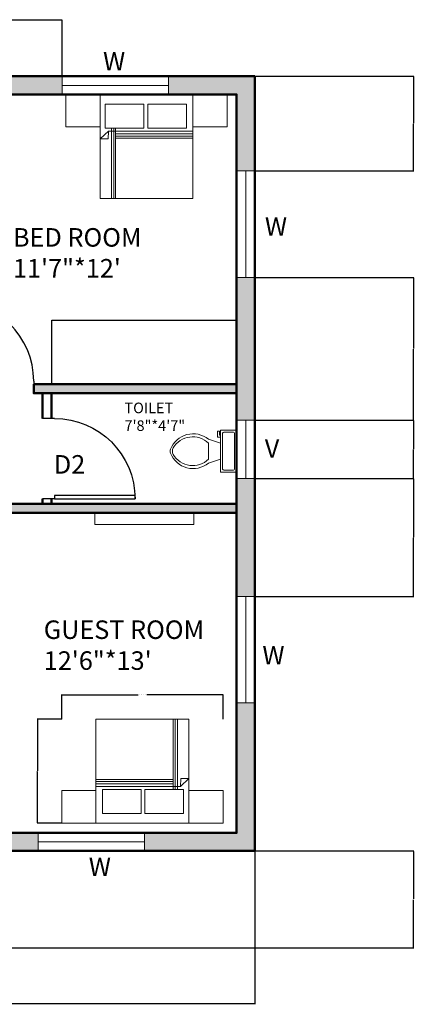
# Model space of a CAD drawing. Units: inches. Extents: x 2116 to 2704, y 2001 to 2561.
# Tile 2 of 2: x 2508 to 2704, y 2001 to 2490. Entities that reach past the tile are written whole.
import ezdxf

# ---------------------------------------------------------------- set-up
doc = ezdxf.new("R2010")
doc.units = ezdxf.units.IN
doc.linetypes.add('ACAD_ISO02W100', pattern=[15, 12, -3])
for name, color, linetype, lineweight in [('A-ANNO-DIMS', 2, 'Continuous', 18), ('A-AREA-IDEN', 70, 'Continuous', 25), ('A-DOOR', 3, 'Continuous', 25), ('A-FLOR-CASE', 9, 'Continuous', 25), ('A-FLOR-FIXT', 9, 'Continuous', 18), ('A-FURN', 40, 'Continuous', 18), ('A-GLAZ', 4, 'Continuous', 20), ('A-GLAZ-HIDN', 4, 'ACAD_ISO02W100', 18), ('A-WALL-PATT', 172, 'Continuous', 13), ('TEXT', 70, 'Continuous', 18), ('TV', 210, 'Continuous', 18), ('WALL', 7, 'Continuous', 50)]:
    doc.layers.add(name, color=color, linetype=linetype, lineweight=lineweight)
doc.styles.get("Standard").update_dxf_attribs({"font": 'arial.ttf'})
doc.dimstyles.get("Standard").update_dxf_attribs({"dimtxt": 0.18, "dimasz": 0.18, "dimexe": 0.18, "dimexo": 0.0625, "dimgap": 0.09, "dimtad": 0, "dimtih": 1, "dimtoh": 1, "dimdec": 4, "dimzin": 0, "dimdsep": 46, "dimtxsty": 'Standard', "dimcen": 0.09, "dimadec": 0, "dimazin": 0, "dimtfac": 1, "dimtdec": 4, "dimtofl": 0, "dimtmove": 0, "dimatfit": 3, "dimfxl": 1, "dimtolj": 1, "dimtzin": 0, "dimarcsym": 0})

# ---------------------------------------------------------------- blocks, each defined once
blk = doc.blocks.new('*U2')
for p, q in [((0, 0), (0, -6)), ((40, 0), (40, -6))]:
    blk.add_line(p, q)
blk.add_lwpolyline([(0, 0), (0, 40), (1.75, 40), (1.75, 0)], close=True)
blk.add_arc((0, 0), 40, 0, 90)
blk = doc.blocks.new('*U4')
for p, q in [((9.5, -6), (9.5, -2)), ((-10, -8.5), (-8, -8.5)), ((-10, -9.5), (-10, -8.5)), ((-7, -9.5), (-10, -9.5)), ((-8, -8.5), (-8, -8)), ((-7, -8), (-7, -9.5)), ((-4, -8), (-6, -14)), ((4, -8), (6, -14)), ((4, -14), (-4, -14))]:
    blk.add_line(p, q)
blk.add_lwpolyline([(10.5, -8), (10.5, 0), (-10.5, 0), (-10.5, -8)], close=True)
for points in [[(-9.5, -2), (-9.5, -6)], [(8.5, -1), (-8.5, -1)], [(-8.5, -7), (8.5, -7)]]:
    blk.add_lwpolyline(points)
for centre, radius, start, end in [((-8.62, -1.88), 0.884, 81.8699, 188.1301), ((8.62, -1.88), 0.884, 351.8699, 98.1301), ((-8.62, -6.12), 0.884, 171.8699, 278.1301), ((8.62, -6.12), 0.884, 261.8699, 8.1301), ((3.52, -21.58), 12.17, 141.4691, 247.9714), ((4.2, -21.82), 11.33, 136.3677, 238.9468), ((-3.52, -21.58), 12.17, 292.0284, 38.5307), ((-4.2, -21.82), 11.33, 301.053, 43.6321), ((0, -27.88), 4, 245.7318, 294.2682), ((0, -29), 4, 254.8605, 285.1395)]:
    blk.add_arc(centre, radius, start, end)
blk = doc.blocks.new('BED-DOUBLE-WITH-NIGHTSTANDS')
for p, q in [((22.66, 34.94), (22.66, 0)), ((23.77, 34.94), (23.77, 0)), ((24.74, 34.94), (24.74, 0)), ((21.16, 33.51), (16.99, 29.58)), ((16.99, 29.58), (21.04, 29.58)), ((21.04, 29.58), (21.16, 33.51)), ((63.16, 33.51), (21.16, 33.51)), ((24.74, 32.21), (63.16, 32.21)), ((24.74, 30.97), (63.16, 30.97)), ((24.74, 30.05), (63.16, 30.05))]:
    blk.add_line(p, q)
for points in [[(16.99, 51.74), (0, 51.74), (0, 35.55), (16.99, 35.55)], [(16.99, 51.74), (63.16, 51.74), (63.16, 0), (16.99, 0)], [(80.15, 51.74), (63.16, 51.74), (63.16, 35.55), (80.15, 35.55)], [(19.62, 46.86), (38.84, 46.86), (38.84, 34.94), (19.62, 34.94)], [(40.77, 46.86), (59.99, 46.86), (59.99, 34.94), (40.77, 34.94)]]:
    blk.add_lwpolyline(points, close=True)
blk = doc.blocks.new('WIN-PLAN-53IN-NOM')
blk.add_line((0, 4.5), (52.88, 4.5))
blk.add_lwpolyline([(0, 9), (52.88, 9), (52.88, 0), (0, 0)], close=True)
blk = doc.blocks.new('*D9')
at = {"layer": 'A-ANNO-DIMS', "color": 0, "lineweight": -2, "transparency": 16777216}
for p, q in [((2528.83, 2142.83), (2528.83, 2154.97)), ((2529.01, 2154.79), (2566.8, 2154.79)), ((2608.8, 2154.79), (2571.02, 2154.79)), ((2608.98, 2142.83), (2608.98, 2154.97))]:
    blk.add_line(p, q, dxfattribs=at)
at = {"layer": 'A-ANNO-DIMS', "color": 0, "lineweight": 100, "transparency": 16777216}
for points in [[(2529.01, 2154.82), (2529.01, 2154.76), (2528.83, 2154.79)], [(2608.8, 2154.82), (2608.8, 2154.76), (2608.98, 2154.79)]]:
    blk.add_solid(points, dxfattribs=at)
at = {"layer": 'Defpoints', "color": 0, "lineweight": 100, "transparency": 16777216}
for p in [(2528.83, 2154.79), (2528.83, 2142.77), (2608.98, 2142.77)]:
    blk.add_point(p, dxfattribs=at)
at = {"layer": 'A-ANNO-DIMS', "color": 0, "transparency": 16777216, "insert": (2568.91, 2154.79), "char_height": 0.18, "attachment_point": 5}
blk.add_mtext('\\A1;BED WITH NIGHTSTANDS 80 TYP.', dxfattribs=at)
blk = doc.blocks.new('*D10')
at = {"layer": 'A-ANNO-DIMS', "color": 0, "lineweight": -2, "transparency": 16777216}
for p, q in [((2528.77, 2142.77), (2516.63, 2142.77)), ((2516.81, 2142.59), (2516.81, 2117.08)), ((2516.81, 2091.21), (2516.81, 2116.72)), ((2528.77, 2091.03), (2516.63, 2091.03))]:
    blk.add_line(p, q, dxfattribs=at)
at = {"layer": 'A-ANNO-DIMS', "color": 0, "lineweight": 100, "transparency": 16777216}
for points in [[(2516.78, 2142.59), (2516.84, 2142.59), (2516.81, 2142.77)], [(2516.78, 2091.21), (2516.84, 2091.21), (2516.81, 2091.03)]]:
    blk.add_solid(points, dxfattribs=at)
at = {"layer": 'Defpoints', "color": 0, "lineweight": 100, "transparency": 16777216}
for p in [(2528.83, 2142.77), (2516.81, 2091.03), (2528.83, 2091.03)]:
    blk.add_point(p, dxfattribs=at)
at = {"layer": 'A-ANNO-DIMS', "color": 0, "transparency": 16777216, "insert": (2516.81, 2116.9), "char_height": 0.18, "attachment_point": 5}
blk.add_mtext('\\A1;52 TYP.', dxfattribs=at)
blk = doc.blocks.new('*D15')
at = {"layer": 'A-ANNO-DIMS', "color": 0, "lineweight": -2, "transparency": 16777216}
for p, q in [((2439.1, 2462.31), (2439.1, 2490.37)), ((2439.28, 2490.19), (2483.65, 2490.19)), ((2528.8, 2490.19), (2484.43, 2490.19)), ((2528.98, 2462.31), (2528.98, 2490.37))]:
    blk.add_line(p, q, dxfattribs=at)
at = {"layer": 'A-ANNO-DIMS', "color": 0, "lineweight": 100, "transparency": 16777216}
for points in [[(2439.28, 2490.22), (2439.28, 2490.16), (2439.1, 2490.19)], [(2528.8, 2490.22), (2528.8, 2490.16), (2528.98, 2490.19)]]:
    blk.add_solid(points, dxfattribs=at)
at = {"layer": 'Defpoints', "color": 0, "lineweight": 100, "transparency": 16777216}
for p in [(2528.98, 2490.19), (2439.1, 2462.24), (2528.98, 2462.24)]:
    blk.add_point(p, dxfattribs=at)
at = {"layer": 'A-ANNO-DIMS', "color": 0, "transparency": 16777216, "insert": (2484.04, 2490.19), "char_height": 0.18, "attachment_point": 5}
blk.add_mtext('\\A1;89.88', dxfattribs=at)
blk = doc.blocks.new('*D16')
at = {"layer": 'A-ANNO-DIMS', "color": 0, "lineweight": -2, "transparency": 16777216}
for p, q in [((2144.72, 2077.18), (2144.72, 2001.04)), ((2624.72, 2077.18), (2624.72, 2001.04)), ((2144.9, 2001.22), (2384.43, 2001.22)), ((2624.54, 2001.22), (2385.01, 2001.22))]:
    blk.add_line(p, q, dxfattribs=at)
at = {"layer": 'A-ANNO-DIMS', "color": 0, "lineweight": 100, "transparency": 16777216}
for points in [[(2144.9, 2001.25), (2144.9, 2001.19), (2144.72, 2001.22)], [(2624.54, 2001.25), (2624.54, 2001.19), (2624.72, 2001.22)]]:
    blk.add_solid(points, dxfattribs=at)
at = {"layer": 'Defpoints', "color": 0, "lineweight": 100, "transparency": 16777216}
for p in [(2144.72, 2077.24), (2624.72, 2077.24), (2624.72, 2001.22)]:
    blk.add_point(p, dxfattribs=at)
at = {"layer": 'A-ANNO-DIMS', "color": 0, "transparency": 16777216, "insert": (2384.72, 2001.22), "char_height": 0.18, "attachment_point": 5}
blk.add_mtext('\\A1;480', dxfattribs=at)
blk = doc.blocks.new('*D17')
at = {"layer": 'A-ANNO-DIMS', "color": 0, "lineweight": -2, "transparency": 16777216}
for p, q in [((2624.78, 2462.24), (2703.85, 2462.24)), ((2703.67, 2462.06), (2703.67, 2438.9)), ((2703.67, 2415.37), (2703.67, 2438.54)), ((2624.78, 2415.19), (2703.85, 2415.19))]:
    blk.add_line(p, q, dxfattribs=at)
at = {"layer": 'A-ANNO-DIMS', "color": 0, "lineweight": 100, "transparency": 16777216}
for points in [[(2703.64, 2462.06), (2703.7, 2462.06), (2703.67, 2462.24)], [(2703.64, 2415.37), (2703.7, 2415.37), (2703.67, 2415.19)]]:
    blk.add_solid(points, dxfattribs=at)
at = {"layer": 'Defpoints', "color": 0, "lineweight": 100, "transparency": 16777216}
for p in [(2624.72, 2462.24), (2703.67, 2462.24), (2624.72, 2415.19)]:
    blk.add_point(p, dxfattribs=at)
at = {"layer": 'A-ANNO-DIMS', "color": 0, "transparency": 16777216, "insert": (2703.67, 2438.72), "char_height": 0.18, "attachment_point": 5}
blk.add_mtext('\\A1;47.05', dxfattribs=at)
blk = doc.blocks.new('*D18')
at = {"layer": 'A-ANNO-DIMS', "color": 0, "lineweight": -2, "transparency": 16777216}
for p, q in [((2624.78, 2362.32), (2703.85, 2362.32)), ((2703.67, 2362.14), (2703.67, 2327.04)), ((2703.67, 2291.59), (2703.67, 2326.68)), ((2624.78, 2291.41), (2703.85, 2291.41))]:
    blk.add_line(p, q, dxfattribs=at)
at = {"layer": 'A-ANNO-DIMS', "color": 0, "lineweight": 100, "transparency": 16777216}
for points in [[(2703.64, 2362.14), (2703.7, 2362.14), (2703.67, 2362.32)], [(2703.64, 2291.59), (2703.7, 2291.59), (2703.67, 2291.41)]]:
    blk.add_solid(points, dxfattribs=at)
at = {"layer": 'Defpoints', "color": 0, "lineweight": 100, "transparency": 16777216}
for p in [(2624.72, 2362.32), (2703.67, 2362.32), (2624.72, 2291.41)]:
    blk.add_point(p, dxfattribs=at)
at = {"layer": 'A-ANNO-DIMS', "color": 0, "transparency": 16777216, "insert": (2703.67, 2326.86), "char_height": 0.18, "attachment_point": 5}
blk.add_mtext('\\A1;70.9', dxfattribs=at)
blk = doc.blocks.new('*D19')
at = {"layer": 'A-ANNO-DIMS', "color": 0, "lineweight": -2, "transparency": 16777216}
for p, q in [((2624.78, 2291.41), (2703.85, 2291.41)), ((2703.67, 2291.23), (2703.67, 2277.06)), ((2703.67, 2262.53), (2703.67, 2276.7)), ((2624.78, 2262.35), (2703.85, 2262.35))]:
    blk.add_line(p, q, dxfattribs=at)
at = {"layer": 'A-ANNO-DIMS', "color": 0, "lineweight": 100, "transparency": 16777216}
for points in [[(2703.64, 2291.23), (2703.7, 2291.23), (2703.67, 2291.41)], [(2703.64, 2262.53), (2703.7, 2262.53), (2703.67, 2262.35)]]:
    blk.add_solid(points, dxfattribs=at)
at = {"layer": 'Defpoints', "color": 0, "lineweight": 100, "transparency": 16777216}
for p in [(2624.72, 2291.41), (2703.67, 2291.41), (2624.72, 2262.35)]:
    blk.add_point(p, dxfattribs=at)
at = {"layer": 'A-ANNO-DIMS', "color": 0, "transparency": 16777216, "insert": (2703.67, 2276.88), "char_height": 0.18, "attachment_point": 5}
blk.add_mtext('\\A1;29.064', dxfattribs=at)
blk = doc.blocks.new('*D20')
at = {"layer": 'A-ANNO-DIMS', "color": 0, "lineweight": -2, "transparency": 16777216}
for p, q in [((2624.78, 2262.35), (2703.85, 2262.35)), ((2703.67, 2262.17), (2703.67, 2233.24)), ((2703.67, 2203.96), (2703.67, 2232.88)), ((2624.78, 2203.78), (2703.85, 2203.78))]:
    blk.add_line(p, q, dxfattribs=at)
at = {"layer": 'A-ANNO-DIMS', "color": 0, "lineweight": 100, "transparency": 16777216}
for points in [[(2703.64, 2262.17), (2703.7, 2262.17), (2703.67, 2262.35)], [(2703.64, 2203.96), (2703.7, 2203.96), (2703.67, 2203.78)]]:
    blk.add_solid(points, dxfattribs=at)
at = {"layer": 'Defpoints', "color": 0, "lineweight": 100, "transparency": 16777216}
for p in [(2624.72, 2262.35), (2703.67, 2262.35), (2624.72, 2203.78)]:
    blk.add_point(p, dxfattribs=at)
at = {"layer": 'A-ANNO-DIMS', "color": 0, "transparency": 16777216, "insert": (2703.67, 2233.06), "char_height": 0.18, "attachment_point": 5}
blk.add_mtext('\\A1;58.57', dxfattribs=at)
blk = doc.blocks.new('*D21')
at = {"layer": 'A-ANNO-DIMS', "color": 0, "lineweight": -2, "transparency": 16777216}
for p, q in [((2624.78, 2077.24), (2703.85, 2077.24)), ((2703.67, 2077.06), (2703.67, 2053.39)), ((2703.67, 2029.35), (2703.67, 2053.03)), ((2413.8, 2029.17), (2703.85, 2029.17))]:
    blk.add_line(p, q, dxfattribs=at)
at = {"layer": 'A-ANNO-DIMS', "color": 0, "lineweight": 100, "transparency": 16777216}
for points in [[(2703.64, 2077.06), (2703.7, 2077.06), (2703.67, 2077.24)], [(2703.64, 2029.35), (2703.7, 2029.35), (2703.67, 2029.17)]]:
    blk.add_solid(points, dxfattribs=at)
at = {"layer": 'Defpoints', "color": 0, "lineweight": 100, "transparency": 16777216}
for p in [(2624.72, 2077.24), (2703.67, 2077.24), (2413.74, 2029.17)]:
    blk.add_point(p, dxfattribs=at)
at = {"layer": 'A-ANNO-DIMS', "color": 0, "transparency": 16777216, "insert": (2703.67, 2053.21), "char_height": 0.18, "attachment_point": 5}
blk.add_mtext('\\A1;48.07', dxfattribs=at)

msp = doc.modelspace()

# ---------------------------------------------------------------- hatches: boundary and pattern name
at = {"layer": 'A-WALL-PATT'}
h = msp.add_hatch(color=256, dxfattribs=at)
h.dxf.hatch_style = 1
h.paths.add_polyline_path([(2187.7856, 2462.2434), (2144.722, 2462.2434), (2144.722, 2419.3525), (2153.722, 2419.3525), (2153.722, 2453.2434), (2187.7856, 2453.2434)])
h.paths.add_polyline_path([(2302.9116, 2462.2434), (2240.6643, 2462.2434), (2240.6643, 2453.2434), (2241.4366, 2453.2434), (2285.722, 2453.2434), (2302.9116, 2453.2434)])
h.paths.add_polyline_path([(2153.722, 2366.4738), (2144.722, 2366.4738), (2144.722, 2275.9883), (2153.722, 2275.9883)])
h.paths.add_polyline_path([(2386.2219, 2462.2434), (2332.038, 2462.2434), (2332.038, 2453.2434), (2344.222, 2453.2434), (2386.2219, 2453.2434)])
h.paths.add_polyline_path([(2528.9791, 2462.2434), (2439.1006, 2462.2434), (2439.1006, 2453.2434), (2528.9791, 2453.2434)])
h.paths.add_polyline_path([(2624.722, 2462.2434), (2581.8578, 2462.2434), (2581.8578, 2453.2434), (2594.0001, 2453.2434), (2610.9949, 2453.2434), (2615.722, 2453.2434), (2615.722, 2415.194), (2624.722, 2415.194)])
h = msp.add_hatch(color=256, dxfattribs=at)
h.dxf.hatch_style = 1
h.paths.add_polyline_path([(2473.222, 2453.2434), (2468.722, 2453.2434), (2468.722, 2309.2434), (2473.222, 2309.2434)])
h.paths.add_polyline_path([(2474.8589, 2309.2434), (2467.2113, 2309.2434), (2467.2113, 2304.7434), (2474.8589, 2304.7434)])
h.paths.add_polyline_path([(2615.722, 2309.2434), (2514.8589, 2309.2434), (2514.8589, 2304.7434), (2615.722, 2304.7434)])
h.paths.add_polyline_path([(2624.722, 2362.3153), (2615.722, 2362.3153), (2615.722, 2309.2434), (2615.722, 2304.7434), (2615.722, 2291.4101), (2624.722, 2291.4101)])
h.paths.add_polyline_path([(2348.722, 2336.7395), (2348.722, 2356.7434), (2344.222, 2356.7434), (2344.222, 2304.7434), (2427.2113, 2304.7434), (2427.2113, 2309.2434), (2348.722, 2309.2434)])
h.paths.add_polyline_path([(2348.722, 2453.2434), (2344.222, 2453.2434), (2344.222, 2361.2434), (2290.222, 2361.2434), (2290.222, 2356.7434), (2348.722, 2356.7434)])
h.paths.add_polyline_path([(2290.222, 2453.2434), (2285.722, 2453.2434), (2285.722, 2404.3805), (2290.222, 2404.3805)])
h.paths.add_polyline_path([(2290.222, 2312.0296), (2285.722, 2312.0296), (2285.722, 2309.2434), (2153.722, 2309.2434), (2153.722, 2304.7434), (2177.722, 2304.7434), (2268.722, 2304.7434), (2290.222, 2304.7434)])
h.paths.add_polyline_path([(2273.222, 2304.7434), (2268.722, 2304.7434), (2268.722, 2301.0301), (2273.222, 2301.0301)])
h = msp.add_hatch(color=256, dxfattribs=at)
h.dxf.hatch_style = 1
h.paths.add_polyline_path([(2406.222, 2179.2434), (2408.2564, 2179.2434), (2408.2564, 2183.7434), (2401.722, 2183.7434), (2401.722, 2086.2434), (2406.222, 2086.2434)])
h.paths.add_polyline_path([(2465.722, 2200.9957), (2461.222, 2200.9957), (2461.222, 2086.2434), (2465.722, 2086.2434)])
h.paths.add_polyline_path([(2461.222, 2183.7434), (2448.2564, 2183.7434), (2448.2564, 2179.2434), (2461.222, 2179.2434)])
h.paths.add_polyline_path([(2401.722, 2183.7434), (2393.523, 2183.7434), (2393.523, 2182.34), (2393.523, 2179.2434), (2401.722, 2179.2434)])
h.paths.add_polyline_path([(2415.304, 2086.2434), (2406.222, 2086.2434), (2401.722, 2086.2434), (2401.722, 2077.2434), (2415.304, 2077.2434)])
h.paths.add_polyline_path([(2298.722, 2086.2434), (2153.722, 2086.2434), (2153.722, 2111.0387), (2144.722, 2111.0387), (2144.722, 2077.2434), (2298.722, 2077.2434)])
h.paths.add_polyline_path([(2360.0446, 2163.1907), (2373.9305, 2163.1907), (2373.9305, 2182.1552), (2360.0446, 2182.1552)], flags=9)
h.paths.add_polyline_path([(2315.961, 2097.9087), (2338.4221, 2097.9087), (2338.4221, 2116.8732), (2315.961, 2116.8732)], flags=9)
h.paths.add_polyline_path([(2316.4397, 2126.7155), (2376.3025, 2126.7155), (2376.3025, 2161.0558), (2316.4397, 2161.0558)], flags=9)
h.paths.add_polyline_path([(2521.5838, 2259.7103), (2542.6199, 2259.7103), (2542.6199, 2278.6748), (2521.5838, 2278.6748)], flags=9)
h.paths.add_polyline_path([(2484.5309, 2304.0263), (2505.567, 2304.0263), (2505.567, 2322.9908), (2484.5309, 2322.9908)], flags=9)
h.paths.add_polyline_path([(2436.5934, 2307.3012), (2457.6295, 2307.3012), (2457.6295, 2326.2657), (2436.5934, 2326.2657)], flags=9)
h.paths.add_polyline_path([(2279.8188, 2377.038), (2300.8549, 2377.038), (2300.8549, 2396.0025), (2279.8188, 2396.0025)], flags=9)
h.paths.add_polyline_path([(2265.2604, 2320.3349), (2286.2965, 2320.3349), (2286.2965, 2339.2994), (2265.2604, 2339.2994)], flags=9)
h.paths.add_polyline_path([(2259.5917, 2272.3677), (2280.6278, 2272.3677), (2280.6278, 2291.3322), (2259.5917, 2291.3322)], flags=9)
h.paths.add_polyline_path([(2466.8383, 2211.6782), (2487.8744, 2211.6782), (2487.8744, 2230.6428), (2466.8383, 2230.6428)], flags=9)
h.paths.add_polyline_path([(2416.3041, 2164.7232), (2437.3402, 2164.7232), (2437.3402, 2183.6877), (2416.3041, 2183.6877)], flags=9)
h.paths.add_polyline_path([(2464.3943, 2274.2881), (2513.2984, 2274.2881), (2513.2984, 2285.1577), (2464.3943, 2285.1577)], flags=9)
h.paths.add_polyline_path([(2558.3191, 2283.0075), (2588.2617, 2283.0075), (2588.2617, 2302.6898), (2558.3191, 2302.6898)], flags=9)
h.paths.add_polyline_path([(2187.7928, 2218.693), (2248.8232, 2218.693), (2248.8232, 2253.0333), (2187.7928, 2253.0333)], flags=9)
h.paths.add_polyline_path([(2407.3216, 2101.5621), (2460.3921, 2101.5621), (2460.3921, 2135.9024), (2407.3216, 2135.9024)], flags=9)
h.paths.add_polyline_path([(2516.1575, 2162.0461), (2609.3291, 2162.0461), (2609.3291, 2196.3865), (2516.1575, 2196.3865)], flags=9)
h.paths.add_polyline_path([(2339.9087, 2244.2645), (2455.623, 2244.2645), (2455.623, 2278.6049), (2339.9087, 2278.6049)], flags=9)
h.paths.add_polyline_path([(2500.8533, 2357.0199), (2575.9141, 2357.0199), (2575.9141, 2391.3602), (2500.8533, 2391.3602)], flags=9)
h.paths.add_polyline_path([(2361.5168, 2352.6691), (2436.5776, 2352.6691), (2436.5776, 2387.0094), (2361.5168, 2387.0094)], flags=9)
h.paths.add_polyline_path([(2310.3217, 2400.2918), (2340.3434, 2400.2918), (2340.3434, 2419.9741), (2310.3217, 2419.9741)], flags=9)
h.paths.add_polyline_path([(2164.0511, 2360.101), (2253.3807, 2360.101), (2253.3807, 2394.4413), (2164.0511, 2394.4413)], flags=9)
h = msp.add_hatch(color=256, dxfattribs=at)
h.dxf.hatch_style = 1
h.paths.add_polyline_path([(2624.722, 2150.901), (2615.722, 2150.901), (2615.722, 2086.2434), (2569.9026, 2086.2434), (2569.9026, 2077.2434), (2624.722, 2077.2434)])
h.paths.add_polyline_path([(2517.0239, 2086.2434), (2465.722, 2086.2434), (2449.7631, 2086.2434), (2449.7631, 2077.2434), (2517.0239, 2077.2434)])
h.paths.add_polyline_path([(2624.722, 2262.3456), (2615.722, 2262.3456), (2615.722, 2249.7434), (2615.722, 2203.7797), (2624.722, 2203.7797)])
h.paths.add_polyline_path([(2521.5838, 2259.7103), (2542.6199, 2259.7103), (2542.6199, 2278.6748), (2521.5838, 2278.6748)], flags=9)
h.paths.add_polyline_path([(2484.5309, 2304.0263), (2505.567, 2304.0263), (2505.567, 2322.9908), (2484.5309, 2322.9908)], flags=9)
h.paths.add_polyline_path([(2436.5934, 2307.3012), (2457.6295, 2307.3012), (2457.6295, 2326.2657), (2436.5934, 2326.2657)], flags=9)
h.paths.add_polyline_path([(2279.8188, 2377.038), (2300.8549, 2377.038), (2300.8549, 2396.0025), (2279.8188, 2396.0025)], flags=9)
h.paths.add_polyline_path([(2265.2604, 2320.3349), (2286.2965, 2320.3349), (2286.2965, 2339.2994), (2265.2604, 2339.2994)], flags=9)
h.paths.add_polyline_path([(2259.5917, 2272.3677), (2280.6278, 2272.3677), (2280.6278, 2291.3322), (2259.5917, 2291.3322)], flags=9)
h.paths.add_polyline_path([(2466.8383, 2211.6782), (2487.8744, 2211.6782), (2487.8744, 2230.6428), (2466.8383, 2230.6428)], flags=9)
h.paths.add_polyline_path([(2416.3041, 2164.7232), (2437.3402, 2164.7232), (2437.3402, 2183.6877), (2416.3041, 2183.6877)], flags=9)
h.paths.add_polyline_path([(2464.3943, 2274.2881), (2513.2984, 2274.2881), (2513.2984, 2285.1577), (2464.3943, 2285.1577)], flags=9)
h.paths.add_polyline_path([(2558.3191, 2283.0075), (2588.2617, 2283.0075), (2588.2617, 2302.6898), (2558.3191, 2302.6898)], flags=9)
h.paths.add_polyline_path([(2187.7928, 2218.693), (2248.8232, 2218.693), (2248.8232, 2253.0333), (2187.7928, 2253.0333)], flags=9)
h.paths.add_polyline_path([(2407.3216, 2101.5621), (2460.3921, 2101.5621), (2460.3921, 2135.9024), (2407.3216, 2135.9024)], flags=9)
h.paths.add_polyline_path([(2516.1575, 2162.0461), (2609.3291, 2162.0461), (2609.3291, 2196.3865), (2516.1575, 2196.3865)], flags=9)
h.paths.add_polyline_path([(2339.9087, 2244.2645), (2455.623, 2244.2645), (2455.623, 2278.6049), (2339.9087, 2278.6049)], flags=9)
h.paths.add_polyline_path([(2500.8533, 2357.0199), (2575.9141, 2357.0199), (2575.9141, 2391.3602), (2500.8533, 2391.3602)], flags=9)
h.paths.add_polyline_path([(2361.5168, 2352.6691), (2436.5776, 2352.6691), (2436.5776, 2387.0094), (2361.5168, 2387.0094)], flags=9)
h.paths.add_polyline_path([(2310.3217, 2400.2918), (2340.3434, 2400.2918), (2340.3434, 2419.9741), (2310.3217, 2419.9741)], flags=9)
h.paths.add_polyline_path([(2164.0511, 2360.101), (2253.3807, 2360.101), (2253.3807, 2394.4413), (2164.0511, 2394.4413)], flags=9)
h = msp.add_hatch(color=256, dxfattribs=at)
h.dxf.hatch_style = 1
h.paths.add_polyline_path([(2615.722, 2249.7434), (2461.222, 2249.7434), (2461.222, 2245.3695), (2465.722, 2245.3695), (2615.722, 2245.3695)])
h.paths.add_polyline_path([(2465.722, 2245.3695), (2461.222, 2245.3695), (2461.222, 2240.9957), (2465.722, 2240.9957)])
h.paths.add_polyline_path([(2153.722, 2223.1096), (2144.722, 2223.1096), (2144.722, 2163.9174), (2153.722, 2163.9174)])
h.paths.add_polyline_path([(2352.235, 2183.7434), (2153.722, 2183.7434), (2153.8615, 2179.2434), (2352.235, 2179.2434), (2352.235, 2182.34)])
h.paths.add_polyline_path([(2273.222, 2261.0301), (2268.722, 2261.0301), (2268.722, 2183.7434), (2273.222, 2183.7434)])

# ---------------------------------------------------------------- linework, layer by layer
at = {"layer": 'A-FLOR-CASE'}
msp.add_lwpolyline([(2615.722, 2309.2434), (2523.8946, 2309.2434), (2523.8946, 2341.0381), (2615.722, 2341.0381)], close=True, dxfattribs=at)
at = {"layer": 'A-GLAZ'}
msp.add_line((2620.222, 2262.3456), (2620.222, 2291.4101), dxfattribs=at)
at = {"layer": 'A-GLAZ-HIDN'}
msp.add_lwpolyline([(2615.722, 2262.3456), (2624.722, 2262.3456), (2624.722, 2291.4101), (2615.722, 2291.4101)], close=True, dxfattribs=at)
at = {"layer": 'TV'}
msp.add_lwpolyline([(2545.233, 2245.2434), (2594.5247, 2245.2434), (2594.5247, 2239.432), (2545.233, 2239.432)], close=True, dxfattribs=at)
at = {"layer": 'WALL'}
for p, q in [((2514.8589, 2309.2434), (2615.722, 2309.2434)), ((2514.8589, 2304.7434), (2615.722, 2304.7434)), ((2519.222, 2292.2152), (2519.222, 2304.7434)), ((2523.722, 2292.2152), (2523.722, 2304.7434)), ((2615.722, 2304.7434), (2615.722, 2249.7434)), ((2519.222, 2249.7434), (2519.222, 2252.2152)), ((2523.722, 2249.7434), (2523.722, 2252.2152)), ((2461.222, 2249.7434), (2519.222, 2249.7434)), ((2615.722, 2249.7434), (2523.722, 2249.7434)), ((2465.722, 2245.2434), (2521.3308, 2245.2434)), ((2615.722, 2245.2434), (2519.222, 2245.2434)), ((2615.722, 2086.2434), (2465.722, 2086.2434))]:
    msp.add_line(p, q, dxfattribs=at)
for points in [[(2401.722, 2077.2434), (2624.722, 2077.2434), (2624.722, 2462.2434), (2144.722, 2462.2434), (2144.722, 2077.2434), (2298.722, 2077.2434)], [(2615.722, 2309.2434), (2615.722, 2453.2434), (2153.722, 2453.2434), (2153.722, 2086.2434), (2298.722, 2086.2434)], [(2401.722, 2086.2434), (2615.722, 2086.2434), (2615.722, 2304.7434)]]:
    msp.add_lwpolyline(points, dxfattribs=at)
for points in [[(2514.8589, 2309.2434), (2615.722, 2309.2434), (2615.722, 2304.7434), (2514.8589, 2304.7434)], [(2615.722, 2249.7434), (2461.222, 2249.7434), (2461.222, 2245.3695), (2615.722, 2245.3695)]]:
    msp.add_lwpolyline(points, close=True, dxfattribs=at)

# ---------------------------------------------------------------- block references
at = {"layer": 'A-DOOR'}
msp.add_blockref('*U2', (2474.8589, 2310.7434), dxfattribs=at)
at = {"layer": 'A-DOOR', "xscale": -1, "rotation": 270}
msp.add_blockref('*U2', (2525.222, 2252.2152), dxfattribs=at)
at = {"layer": 'A-FLOR-FIXT', "rotation": 270}
msp.add_blockref('*U4', (2615.722, 2275.9281), dxfattribs=at)
at = {"layer": 'A-FURN'}
msp.add_blockref('BED-DOUBLE-WITH-NIGHTSTANDS', (2530.8414, 2401.5064), dxfattribs=at)
at = {"layer": 'A-FURN', "rotation": 180}
msp.add_blockref('BED-DOUBLE-WITH-NIGHTSTANDS', (2608.9843, 2142.7703), dxfattribs=at)
at = {"layer": 'A-GLAZ'}
for p in [(2528.9791, 2453.2434), (2517.0239, 2077.2434)]:
    msp.add_blockref('WIN-PLAN-53IN-NOM', p, dxfattribs=at)
at = {"layer": 'A-GLAZ', "rotation": 270.0000000000007}
for p in [(2615.722, 2415.194), (2615.722, 2203.7797)]:
    msp.add_blockref('WIN-PLAN-53IN-NOM', p, dxfattribs=at)

# ---------------------------------------------------------------- texts
at = {"layer": 'A-AREA-IDEN', "attachment_point": 1}
for s, width, gutter_width, insert, char_height in [('BED ROOM\\P11\'7"*12\'', 294.496073, 46.0145, (2504.5539, 2386.787), 9.2029), ('TOILET\\P7\'8"*4\'7"', 168.791536, 26.3734, (2559.9868, 2300.0687), 5.27468), ('GUEST ROOM\\P12\'6"*13\'', 294.496073, 46.0145, (2519.8581, 2191.8133), 9.2029)]:
    msp.add_mtext_dynamic_manual_height_columns(s, width=width, gutter_width=gutter_width, heights=[0], dxfattribs=dict(at, insert=insert, char_height=char_height))
at = {"layer": 'TEXT', "char_height": 9.2029, "attachment_point": 1}
for s, insert in [('W', (2549.3334, 2474.3449)), ('W', (2629.7785, 2392.1911)), ('V', (2629.7134, 2281.8966)), ('D2', (2524.8763, 2273.976)), ('W', (2628.5312, 2179.1256)), ('W', (2542.229, 2073.9921))]:
    msp.add_mtext_dynamic_manual_height_columns(s, width=294.496073, gutter_width=46.0145, heights=[0], dxfattribs=dict(at, insert=insert))

# ---------------------------------------------------------------- dimensions: what is measured, and where the dimension line sits
at = {"layer": 'A-ANNO-DIMS'}
for base, p1, p2, override, picture, middle in [((2528.9791, 2490.1934), (2439.1006, 2462.2434), (2528.9791, 2462.2434), {"dimdec": 2, "dimlfac": 1, "dimrnd": 0, "dimzin": 0, "dimdsep": 46, "dimlunit": 2}, '*D15', (2484.0398, 2490.1934)), ((2624.722, 2001.2238), (2144.722, 2077.2434), (2624.722, 2077.2434), {"dimdec": 0, "dimlfac": 1, "dimrnd": 0, "dimzin": 0, "dimdsep": 46, "dimlunit": 2}, '*D16', (2384.722, 2001.2238))]:
    dim = msp.add_linear_dim(base=base, p1=p1, p2=p2, dimstyle='Standard', override=override, dxfattribs=at)
    dim.commit()
    dim.dimension.update_dxf_attribs({"geometry": picture, "text_midpoint": middle})
for base, p1, p2, override, picture, middle in [((2703.672, 2462.2434), (2624.722, 2415.194), (2624.722, 2462.2434), {"dimdec": 2, "dimlfac": 1, "dimrnd": 0, "dimzin": 0, "dimdsep": 46, "dimlunit": 2}, '*D17', (2703.672, 2438.7187)), ((2703.672, 2362.3153), (2624.722, 2291.4101), (2624.722, 2362.3153), {"dimdec": 1, "dimlfac": 1, "dimrnd": 0, "dimzin": 0, "dimdsep": 46, "dimlunit": 2}, '*D18', (2703.672, 2326.8627)), ((2703.672002, 2291.410059), (2624.722002, 2262.345563), (2624.722002, 2291.410059), {"dimdec": 3, "dimlfac": 1, "dimrnd": 0, "dimzin": 0, "dimdsep": 46, "dimlunit": 2}, '*D19', (2703.672002, 2276.877811)), ((2703.672, 2262.3456), (2624.722, 2203.7797), (2624.722, 2262.3456), {"dimdec": 2, "dimlfac": 1, "dimrnd": 0, "dimzin": 0, "dimdsep": 46, "dimlunit": 2}, '*D20', (2703.672, 2233.0626)), ((2703.672, 2077.2434), (2413.7384, 2029.1738), (2624.722, 2077.2434), {"dimdec": 2, "dimlfac": 1, "dimrnd": 0, "dimzin": 0, "dimdsep": 46, "dimlunit": 2}, '*D21', (2703.672, 2053.2086))]:
    dim = msp.add_linear_dim(base=base, p1=p1, p2=p2, angle=90, dimstyle='Standard', override=override, dxfattribs=at)
    dim.commit()
    dim.dimension.update_dxf_attribs({"geometry": picture, "text_midpoint": middle})
for base, p1, p2, angle, text, picture, middle in [((2528.8308, 2154.7934), (2608.9843, 2142.7703), (2528.8308, 2142.7703), 180, 'BED WITH NIGHTSTANDS <> TYP.', '*D9', (2568.9076, 2154.7934)), ((2516.8078, 2091.0334), (2528.8308, 2142.7703), (2528.8308, 2091.0334), 270, '<> TYP.', '*D10', (2516.8078, 2116.9018))]:
    dim = msp.add_linear_dim(base=base, p1=p1, p2=p2, angle=angle, text=text, dimstyle='Standard', override={"dimdec": 0, "dimlfac": 1, "dimrnd": 0, "dimzin": 0, "dimdsep": 46, "dimlunit": 2}, dxfattribs=at)
    dim.commit()
    dim.dimension.update_dxf_attribs({"geometry": picture, "text_midpoint": middle})

doc.saveas('drawing.dxf')
